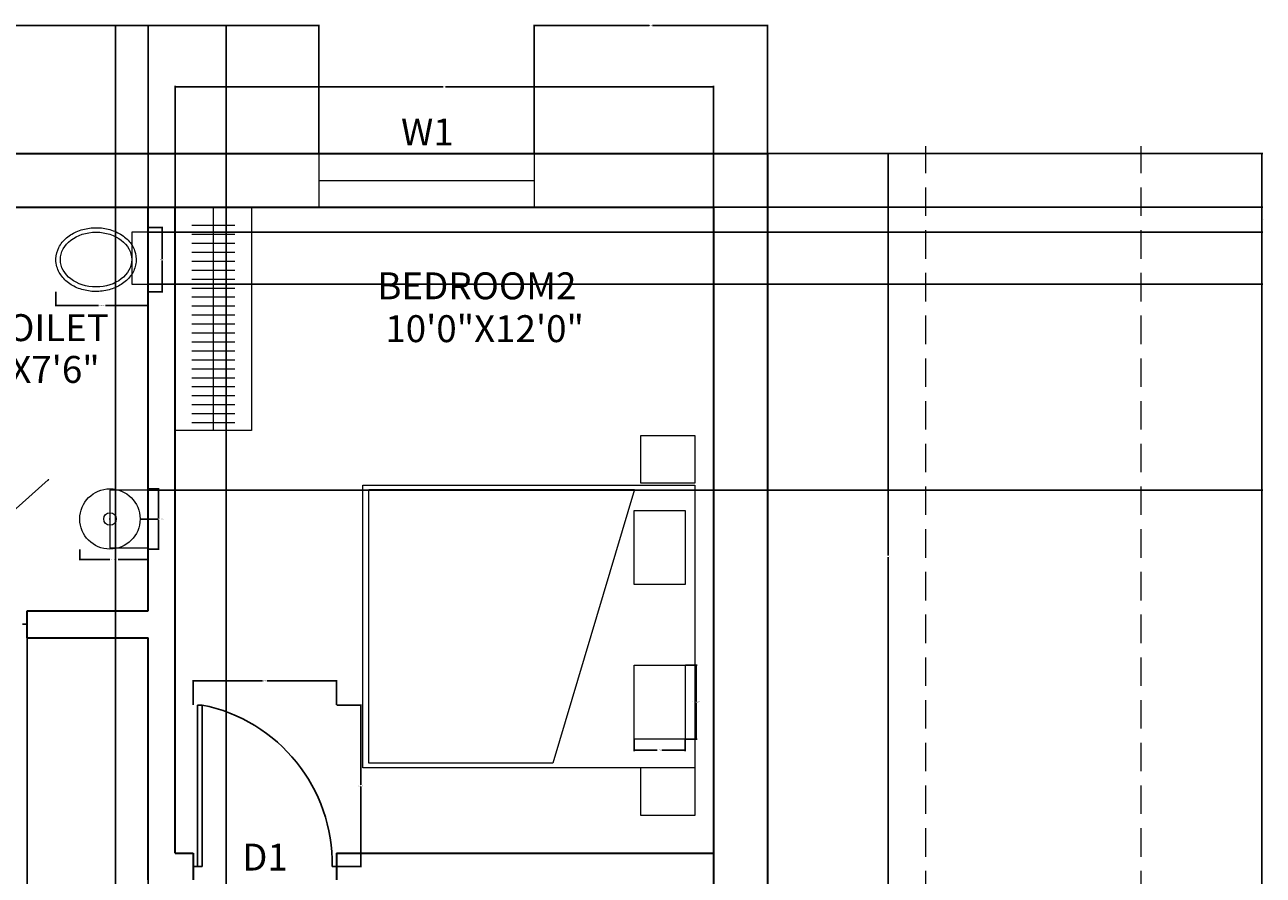
# Model space of a CAD drawing. Units: inches. Extents: x 2906 to 3403, y 1614 to 2150.
# Tile 4 of 4: x 3127 to 3403, y 1960 to 2150. Entities that reach past the tile are written whole.
import ezdxf

# ---------------------------------------------------------------- set-up
doc = ezdxf.new("R2010")
doc.units = ezdxf.units.IN
doc.linetypes.add('DASHED2', pattern=[9.525, 6.35, -3.175])
for name, color, linetype, lineweight in [('A-ANNO-DIMS', 2, 'Continuous', 18), ('A-ANNO-TEXT', 220, 'Continuous', 18), ('A-AREA-IDEN', 220, 'Continuous', 25), ('A-DOOR', 40, 'Continuous', 25), ('A-FLOR-CASE', 121, 'Continuous', 18), ('A-FLOR-FIXT', 121, 'Continuous', 18), ('A-FURN', 121, 'Continuous', 18), ('A-GLAZ', 2, 'Continuous', 18), ('A-WALL', 191, 'Continuous', 35), ('C-ROAD', 255, 'DASHED2', 18)]:
    doc.layers.add(name, color=color, linetype=linetype, lineweight=lineweight)
doc.styles.get("Standard").update_dxf_attribs({"font": 'arial.ttf'})
doc.dimstyles.get("Standard").update_dxf_attribs({"dimtxt": 0.18, "dimasz": 0.18, "dimexe": 0.18, "dimexo": 0.0625, "dimgap": 0.09, "dimtad": 0, "dimtih": 1, "dimtoh": 1, "dimdec": 4, "dimzin": 0, "dimdsep": 46, "dimtxsty": 'Standard', "dimcen": 0.09, "dimadec": 0, "dimazin": 0, "dimtfac": 1, "dimtdec": 4, "dimtofl": 0, "dimtmove": 0, "dimatfit": 3, "dimfxl": 1, "dimtolj": 1, "dimtzin": 0, "dimarcsym": 0})

# ---------------------------------------------------------------- blocks, each defined once
blk = doc.blocks.new('DOOR-SWING-36')
for p, q in [((36, 32), (36, 31)), ((0, 1), (0, 2)), ((0, 2), (36, 2)), ((36, 1), (0, 1)), ((36, 2), (36, 1)), ((36, 0), (36, 1))]:
    blk.add_line(p, q)
blk.add_arc((35.31, -4.99), 36, 88.9084, 168.7983)
blk = doc.blocks.new('WINDOW-48')
for p, q in [((0, 12), (0, 0)), ((48, 12), (48, 0)), ((0, 6), (48, 6))]:
    blk.add_line(p, q)
blk = doc.blocks.new('WC-FLOOR')
blk.add_lwpolyline([(20.57, 13.25), (16.9, 13.25), (16.9, 1.66), (20.57, 1.66)], close=True)
blk.add_ellipse((8.95, 7.12), major_axis=(-7.95, 0), ratio=0.769471)
blk.add_open_spline([(0, 7.12), (0, 6.57), (0.08, 6.02), (0.48, 4.65), (0.93, 3.84), (2.12, 2.43), (2.86, 1.82), (4.56, 0.85), (5.51, 0.49), (7.5, 0.04), (8.54, -0.04), (10.6, 0.07), (11.62, 0.27), (13.52, 0.93), (14.4, 1.4), (15.92, 2.56), (16.56, 3.25), (17.49, 4.8), (17.78, 5.66), (17.96, 7.41), (17.85, 8.3), (17.23, 9.97), (16.74, 10.74), (15.46, 12.09), (14.67, 12.67), (12.92, 13.56), (11.94, 13.88), (9.93, 14.24), (8.88, 14.28), (6.83, 14.08), (5.83, 13.84), (3.97, 13.1), (3.12, 12.59), (1.68, 11.37), (1.09, 10.64), (0.26, 9.05), (0.03, 8.17), (0, 7.24), (0, 7.18), (0, 7.12)], degree=3, knots=[0, 0, 0, 0, 0.221105, 0.221105, 0.576279, 0.576279, 0.931454, 0.931454, 1.286628, 1.286628, 1.641803, 1.641803, 1.996977, 1.996977, 2.352152, 2.352152, 2.707326, 2.707326, 3.062501, 3.062501, 3.417675, 3.417675, 3.77285, 3.77285, 4.128024, 4.128024, 4.483198, 4.483198, 4.838373, 4.838373, 5.193547, 5.193547, 5.548722, 5.548722, 5.903896, 5.903896, 6.259071, 6.259071, 6.283185, 6.283185, 6.283185, 6.283185])
blk = doc.blocks.new('LAVATORY-WALL')
blk.add_lwpolyline([(15.24, 13.17), (6.72, 13.17), (6.72, 0.27), (15.24, 0.27)], close=True)
for radius in [6.72, 1.39]:
    blk.add_circle((6.72, 6.72), radius)
blk = doc.blocks.new('WARDROBE-RAIL')
for p, q in [((4.8, 49.77), (4.8, 0)), ((0, 45.77), (9.61, 45.77)), ((0, 43.77), (9.61, 43.77)), ((0, 41.77), (9.61, 41.77)), ((0, 39.77), (9.61, 39.77)), ((0, 37.77), (9.61, 37.77)), ((0, 35.77), (9.61, 35.77)), ((0, 33.77), (9.61, 33.77)), ((0, 31.77), (9.61, 31.77)), ((0, 29.77), (9.61, 29.77)), ((0, 27.77), (9.61, 27.77)), ((0, 25.77), (9.61, 25.77)), ((0, 23.77), (9.61, 23.77)), ((0, 21.77), (9.61, 21.77)), ((0, 19.77), (9.61, 19.77)), ((0, 17.77), (9.61, 17.77)), ((0, 15.77), (9.61, 15.77)), ((0, 13.77), (9.61, 13.77)), ((0, 11.77), (9.61, 11.77)), ((0, 9.77), (9.61, 9.77)), ((0, 7.77), (9.61, 7.77)), ((0, 5.77), (9.61, 5.77)), ((0, 3.77), (9.61, 3.77)), ((0, 1.77), (9.61, 1.77))]:
    blk.add_line(p, q)
blk = doc.blocks.new('NIGHTSTAND')
blk.add_lwpolyline([(0, 10.63), (12.01, 10.63), (12.01, 0), (0, 0)], close=True)
blk = doc.blocks.new('BED-PILLOW')
blk.add_lwpolyline([(0, 16.48), (11.36, 16.48), (11.36, 0), (0, 0)], close=True)
blk = doc.blocks.new('*D16')
at = {"layer": 'A-ANNO-DIMS', "color": 0, "lineweight": -2, "transparency": 16777216}
for p, q in [((3274.36, 2007.13), (3276.95, 2007.13)), ((3276.77, 2006.95), (3276.77, 1999.07)), ((3276.77, 1990.83), (3276.77, 1998.71)), ((3274.36, 1990.65), (3276.95, 1990.65))]:
    blk.add_line(p, q, dxfattribs=at)
at = {"layer": 'A-ANNO-DIMS', "color": 0, "transparency": 16777216}
for points in [[(3276.74, 2006.95), (3276.8, 2006.95), (3276.77, 2007.13)], [(3276.74, 1990.83), (3276.8, 1990.83), (3276.77, 1990.65)]]:
    blk.add_solid(points, dxfattribs=at)
at = {"layer": 'Defpoints', "color": 0, "transparency": 16777216}
for p in [(3274.3, 2007.13), (3276.77, 2007.13), (3274.3, 1990.65)]:
    blk.add_point(p, dxfattribs=at)
at = {"layer": 'A-ANNO-DIMS', "color": 0, "transparency": 16777216, "insert": (3276.77, 1998.89), "char_height": 0.18, "attachment_point": 5}
blk.add_mtext('\\A1;PILLOW 16 TYP.', dxfattribs=at)
blk = doc.blocks.new('*D17')
at = {"layer": 'A-ANNO-DIMS', "color": 0, "lineweight": -2, "transparency": 16777216}
for p, q in [((3262.93, 1990.59), (3262.93, 1988)), ((3274.3, 1990.59), (3274.3, 1988)), ((3263.11, 1988.18), (3268.1, 1988.18)), ((3274.12, 1988.18), (3269.14, 1988.18))]:
    blk.add_line(p, q, dxfattribs=at)
at = {"layer": 'A-ANNO-DIMS', "color": 0, "transparency": 16777216}
for points in [[(3263.11, 1988.21), (3263.11, 1988.15), (3262.93, 1988.18)], [(3274.12, 1988.21), (3274.12, 1988.15), (3274.3, 1988.18)]]:
    blk.add_solid(points, dxfattribs=at)
at = {"layer": 'Defpoints', "color": 0, "transparency": 16777216}
for p in [(3262.93, 1990.65), (3274.3, 1990.65), (3274.3, 1988.18)]:
    blk.add_point(p, dxfattribs=at)
at = {"layer": 'A-ANNO-DIMS', "color": 0, "transparency": 16777216, "insert": (3268.62, 1988.18), "char_height": 0.18, "attachment_point": 5}
blk.add_mtext('\\A1;11 TYP.', dxfattribs=at)
blk = doc.blocks.new('*D20')
at = {"layer": 'A-ANNO-DIMS', "color": 0, "lineweight": -2, "transparency": 16777216}
for p, q in [((3196.7, 1998.25), (3202.21, 1998.25)), ((3202.03, 1998.07), (3202.03, 1980.44)), ((3202.03, 1962.43), (3202.03, 1980.07)), ((3196.7, 1962.25), (3202.21, 1962.25))]:
    blk.add_line(p, q, dxfattribs=at)
at = {"layer": 'A-ANNO-DIMS', "color": 0, "transparency": 16777216}
for points in [[(3202, 1998.07), (3202.06, 1998.07), (3202.03, 1998.25)], [(3202, 1962.43), (3202.06, 1962.43), (3202.03, 1962.25)]]:
    blk.add_solid(points, dxfattribs=at)
at = {"layer": 'Defpoints', "color": 0, "transparency": 16777216}
for p in [(3196.63, 1998.25), (3196.63, 1962.25), (3202.03, 1962.25)]:
    blk.add_point(p, dxfattribs=at)
at = {"layer": 'A-ANNO-DIMS', "color": 0, "transparency": 16777216, "insert": (3202.03, 1980.25), "char_height": 0.18, "attachment_point": 5}
blk.add_mtext('\\A1;D1 36 TYP.', dxfattribs=at)
blk = doc.blocks.new('*D21')
at = {"layer": 'A-ANNO-DIMS', "color": 0, "lineweight": -2, "transparency": 16777216}
for p, q in [((3164.63, 1998.32), (3164.63, 2003.83)), ((3196.63, 1998.32), (3196.63, 2003.83)), ((3164.81, 2003.65), (3180.1, 2003.65)), ((3196.45, 2003.65), (3181.16, 2003.65))]:
    blk.add_line(p, q, dxfattribs=at)
at = {"layer": 'A-ANNO-DIMS', "color": 0, "transparency": 16777216}
for points in [[(3164.81, 2003.68), (3164.81, 2003.62), (3164.63, 2003.65)], [(3196.45, 2003.68), (3196.45, 2003.62), (3196.63, 2003.65)]]:
    blk.add_solid(points, dxfattribs=at)
at = {"layer": 'Defpoints', "color": 0, "transparency": 16777216}
for p in [(3196.63, 2003.65), (3164.63, 1998.25), (3196.63, 1998.25)]:
    blk.add_point(p, dxfattribs=at)
at = {"layer": 'A-ANNO-DIMS', "color": 0, "transparency": 16777216, "insert": (3180.63, 2003.65), "char_height": 0.18, "attachment_point": 5}
blk.add_mtext('\\A1;32 TYP.', dxfattribs=at)
blk = doc.blocks.new('*D26')
at = {"layer": 'A-ANNO-DIMS', "color": 0, "lineweight": -2, "transparency": 16777216}
for p, q in [((3134.07, 2090.37), (3134.07, 2087.17)), ((3154.63, 2090.37), (3154.63, 2087.17)), ((3134.25, 2087.35), (3143.57, 2087.35)), ((3154.45, 2087.35), (3145.13, 2087.35))]:
    blk.add_line(p, q, dxfattribs=at)
at = {"layer": 'A-ANNO-DIMS', "color": 0, "transparency": 16777216}
for points in [[(3134.25, 2087.38), (3134.25, 2087.32), (3134.07, 2087.35)], [(3154.45, 2087.38), (3154.45, 2087.32), (3154.63, 2087.35)]]:
    blk.add_solid(points, dxfattribs=at)
at = {"layer": 'Defpoints', "color": 0, "transparency": 16777216}
for p in [(3134.07, 2090.43), (3154.63, 2090.43), (3154.63, 2087.35)]:
    blk.add_point(p, dxfattribs=at)
at = {"layer": 'A-ANNO-DIMS', "color": 0, "transparency": 16777216, "insert": (3144.35, 2087.35), "char_height": 0.18, "attachment_point": 5}
blk.add_mtext('\\A1;WC 21 TYP.', dxfattribs=at)
blk = doc.blocks.new('*D27')
at = {"layer": 'A-ANNO-DIMS', "color": 0, "lineweight": -2, "transparency": 16777216}
for p, q in [((3154.7, 2104.76), (3157.9, 2104.76)), ((3157.72, 2104.58), (3157.72, 2097.78)), ((3157.72, 2090.61), (3157.72, 2097.42)), ((3154.7, 2090.43), (3157.9, 2090.43))]:
    blk.add_line(p, q, dxfattribs=at)
at = {"layer": 'A-ANNO-DIMS', "color": 0, "transparency": 16777216}
for points in [[(3157.69, 2104.58), (3157.75, 2104.58), (3157.72, 2104.76)], [(3157.69, 2090.61), (3157.75, 2090.61), (3157.72, 2090.43)]]:
    blk.add_solid(points, dxfattribs=at)
at = {"layer": 'Defpoints', "color": 0, "transparency": 16777216}
for p in [(3154.63, 2104.76), (3157.72, 2104.76), (3154.63, 2090.43)]:
    blk.add_point(p, dxfattribs=at)
at = {"layer": 'A-ANNO-DIMS', "color": 0, "transparency": 16777216, "insert": (3157.72, 2097.6), "char_height": 0.18, "attachment_point": 5}
blk.add_mtext('\\A1;14 TYP.', dxfattribs=at)
blk = doc.blocks.new('*D28')
at = {"layer": 'A-ANNO-DIMS', "color": 0, "lineweight": -2, "transparency": 16777216}
for p, q in [((3139.39, 2032.96), (3139.39, 2030.56)), ((3154.63, 2032.96), (3154.63, 2030.56)), ((3139.57, 2030.74), (3146.08, 2030.74)), ((3154.45, 2030.74), (3147.95, 2030.74))]:
    blk.add_line(p, q, dxfattribs=at)
at = {"layer": 'A-ANNO-DIMS', "color": 0, "transparency": 16777216}
for points in [[(3139.57, 2030.77), (3139.57, 2030.71), (3139.39, 2030.74)], [(3154.45, 2030.77), (3154.45, 2030.71), (3154.63, 2030.74)]]:
    blk.add_solid(points, dxfattribs=at)
at = {"layer": 'Defpoints', "color": 0, "transparency": 16777216}
for p in [(3139.39, 2033.03), (3154.63, 2033.03), (3154.63, 2030.74)]:
    blk.add_point(p, dxfattribs=at)
at = {"layer": 'A-ANNO-DIMS', "color": 0, "transparency": 16777216, "insert": (3147.01, 2030.74), "char_height": 0.18, "attachment_point": 5}
blk.add_mtext('\\A1;BASIN 15 TYP.', dxfattribs=at)
blk = doc.blocks.new('*D29')
at = {"layer": 'A-ANNO-DIMS', "color": 0, "lineweight": -2, "transparency": 16777216}
for p, q in [((3154.7, 2046.46), (3157.1, 2046.46)), ((3156.92, 2046.28), (3156.92, 2039.93)), ((3156.92, 2033.21), (3156.92, 2039.56)), ((3154.7, 2033.03), (3157.1, 2033.03))]:
    blk.add_line(p, q, dxfattribs=at)
at = {"layer": 'A-ANNO-DIMS', "color": 0, "transparency": 16777216}
for points in [[(3156.89, 2046.28), (3156.95, 2046.28), (3156.92, 2046.46)], [(3156.89, 2033.21), (3156.95, 2033.21), (3156.92, 2033.03)]]:
    blk.add_solid(points, dxfattribs=at)
at = {"layer": 'Defpoints', "color": 0, "transparency": 16777216}
for p in [(3154.63, 2046.46), (3156.92, 2046.46), (3154.63, 2033.03)]:
    blk.add_point(p, dxfattribs=at)
at = {"layer": 'A-ANNO-DIMS', "color": 0, "transparency": 16777216, "insert": (3156.92, 2039.74), "char_height": 0.18, "attachment_point": 5}
blk.add_mtext('\\A1;13 TYP.', dxfattribs=at)
blk = doc.blocks.new('*D41')
at = {"layer": 'A-ANNO-DIMS', "color": 0, "lineweight": -2, "transparency": 16777216}
for p, q in [((3292.7, 2121.25), (3403.01, 2121.25)), ((3402.83, 2121.07), (3402.83, 1881.44)), ((3402.83, 1641.43), (3402.83, 1881.07)), ((3292.7, 1641.25), (3403.01, 1641.25))]:
    blk.add_line(p, q, dxfattribs=at)
at = {"layer": 'A-ANNO-DIMS', "color": 0, "transparency": 16777216}
for points in [[(3402.8, 2121.07), (3402.86, 2121.07), (3402.83, 2121.25)], [(3402.8, 1641.43), (3402.86, 1641.43), (3402.83, 1641.25)]]:
    blk.add_solid(points, dxfattribs=at)
at = {"layer": 'Defpoints', "color": 0, "transparency": 16777216}
for p in [(3292.63, 2121.25), (3402.83, 2121.25), (3292.63, 1641.25)]:
    blk.add_point(p, dxfattribs=at)
at = {"layer": 'A-ANNO-DIMS', "color": 0, "transparency": 16777216, "insert": (3402.83, 1881.25), "char_height": 0.18, "attachment_point": 5}
blk.add_mtext('\\A1;480', dxfattribs=at)
blk = doc.blocks.new('*D43')
at = {"layer": 'A-ANNO-DIMS', "color": 0, "lineweight": -2, "transparency": 16777216}
for p, q in [((3025.57, 2121.32), (3025.57, 2149.96)), ((3025.75, 2149.78), (3108.75, 2149.78)), ((3192.49, 2149.78), (3109.49, 2149.78)), ((3192.67, 2121.32), (3192.67, 2149.96))]:
    blk.add_line(p, q, dxfattribs=at)
at = {"layer": 'A-ANNO-DIMS', "color": 0, "transparency": 16777216}
for points in [[(3025.75, 2149.81), (3025.75, 2149.75), (3025.57, 2149.78)], [(3192.49, 2149.81), (3192.49, 2149.75), (3192.67, 2149.78)]]:
    blk.add_solid(points, dxfattribs=at)
at = {"layer": 'Defpoints', "color": 0, "transparency": 16777216}
for p in [(3192.67, 2149.78), (3025.57, 2121.25), (3192.67, 2121.25)]:
    blk.add_point(p, dxfattribs=at)
at = {"layer": 'A-ANNO-DIMS', "color": 0, "transparency": 16777216, "insert": (3109.12, 2149.78), "char_height": 0.18, "attachment_point": 5}
blk.add_mtext('\\A1;167.1', dxfattribs=at)
blk = doc.blocks.new('*D44')
at = {"layer": 'A-ANNO-DIMS', "color": 0, "lineweight": -2, "transparency": 16777216}
for p, q in [((3240.67, 2121.32), (3240.67, 2149.96)), ((3240.85, 2149.78), (3266.26, 2149.78)), ((3292.45, 2149.78), (3267.05, 2149.78)), ((3292.63, 2121.32), (3292.63, 2149.96))]:
    blk.add_line(p, q, dxfattribs=at)
at = {"layer": 'A-ANNO-DIMS', "color": 0, "transparency": 16777216}
for points in [[(3240.85, 2149.81), (3240.85, 2149.75), (3240.67, 2149.78)], [(3292.45, 2149.81), (3292.45, 2149.75), (3292.63, 2149.78)]]:
    blk.add_solid(points, dxfattribs=at)
at = {"layer": 'Defpoints', "color": 0, "transparency": 16777216}
for p in [(3292.63, 2149.78), (3240.67, 2121.25), (3292.63, 2121.25)]:
    blk.add_point(p, dxfattribs=at)
at = {"layer": 'A-ANNO-DIMS', "color": 0, "transparency": 16777216, "insert": (3266.65, 2149.78), "char_height": 0.18, "attachment_point": 5}
blk.add_mtext('\\A1;51.96', dxfattribs=at)
blk = doc.blocks.new('*D46')
at = {"layer": 'A-ANNO-DIMS', "color": 0, "lineweight": -2, "transparency": 16777216}
for p, q in [((3094.63, 2109.32), (3094.63, 2149.96)), ((3094.81, 2149.78), (3124.41, 2149.78)), ((3154.45, 2149.78), (3124.85, 2149.78)), ((3154.63, 2109.32), (3154.63, 2149.96))]:
    blk.add_line(p, q, dxfattribs=at)
at = {"layer": 'A-ANNO-DIMS', "color": 0, "transparency": 16777216}
for points in [[(3094.81, 2149.81), (3094.81, 2149.75), (3094.63, 2149.78)], [(3154.45, 2149.81), (3154.45, 2149.75), (3154.63, 2149.78)]]:
    blk.add_solid(points, dxfattribs=at)
at = {"layer": 'Defpoints', "color": 0, "transparency": 16777216}
for p in [(3154.63, 2149.78), (3094.63, 2109.25), (3154.63, 2109.25)]:
    blk.add_point(p, dxfattribs=at)
at = {"layer": 'A-ANNO-DIMS', "color": 0, "transparency": 16777216, "insert": (3124.63, 2149.78), "char_height": 0.18, "attachment_point": 5}
blk.add_mtext('\\A1;60', dxfattribs=at)
blk = doc.blocks.new('*D47')
at = {"layer": 'A-ANNO-DIMS', "color": 0, "lineweight": -2, "transparency": 16777216}
for p, q in [((3160.63, 2109.32), (3160.63, 2136.33)), ((3280.63, 2109.32), (3280.63, 2136.33)), ((3160.81, 2136.15), (3220.35, 2136.15)), ((3280.45, 2136.15), (3220.91, 2136.15))]:
    blk.add_line(p, q, dxfattribs=at)
at = {"layer": 'A-ANNO-DIMS', "color": 0, "transparency": 16777216}
for points in [[(3160.81, 2136.18), (3160.81, 2136.12), (3160.63, 2136.15)], [(3280.45, 2136.18), (3280.45, 2136.12), (3280.63, 2136.15)]]:
    blk.add_solid(points, dxfattribs=at)
at = {"layer": 'Defpoints', "color": 0, "transparency": 16777216}
for p in [(3280.63, 2136.15), (3160.63, 2109.25), (3280.63, 2109.25)]:
    blk.add_point(p, dxfattribs=at)
at = {"layer": 'A-ANNO-DIMS', "color": 0, "transparency": 16777216, "insert": (3220.63, 2136.15), "char_height": 0.18, "attachment_point": 5}
blk.add_mtext('\\A1;120', dxfattribs=at)
blk = doc.blocks.new('*D66')
at = {"layer": 'A-ANNO-DIMS', "color": 0, "lineweight": -2, "transparency": 16777216}
for p, q in [((3292.7, 2121.25), (3319.71, 2121.25)), ((3319.53, 2121.07), (3319.53, 2031.6)), ((3319.53, 1941.76), (3319.53, 2031.24)), ((3292.7, 1941.58), (3319.71, 1941.58))]:
    blk.add_line(p, q, dxfattribs=at)
at = {"layer": 'A-ANNO-DIMS', "color": 0, "transparency": 16777216}
for points in [[(3319.5, 2121.07), (3319.56, 2121.07), (3319.53, 2121.25)], [(3319.5, 1941.76), (3319.56, 1941.76), (3319.53, 1941.58)]]:
    blk.add_solid(points, dxfattribs=at)
at = {"layer": 'Defpoints', "color": 0, "transparency": 16777216}
for p in [(3292.63, 2121.25), (3292.63, 1941.58), (3319.53, 1941.58)]:
    blk.add_point(p, dxfattribs=at)
at = {"layer": 'A-ANNO-DIMS', "color": 0, "transparency": 16777216, "insert": (3319.53, 2031.42), "char_height": 0.18, "attachment_point": 5}
blk.add_mtext('\\A1;179.67', dxfattribs=at)
blk = doc.blocks.new('*D75')
at = {"layer": 'A-ANNO-DIMS', "color": 0, "lineweight": -2, "transparency": 16777216}
for p, q in [((3127.63, 2013.19), (3127.63, 1613.51)), ((3154.63, 2013.19), (3154.63, 1613.51)), ((3127.81, 1613.69), (3140.91, 1613.69)), ((3154.45, 1613.69), (3141.35, 1613.69))]:
    blk.add_line(p, q, dxfattribs=at)
at = {"layer": 'A-ANNO-DIMS', "color": 0, "transparency": 16777216}
for points in [[(3127.81, 1613.72), (3127.81, 1613.66), (3127.63, 1613.69)], [(3154.45, 1613.72), (3154.45, 1613.66), (3154.63, 1613.69)]]:
    blk.add_solid(points, dxfattribs=at)
at = {"layer": 'Defpoints', "color": 0, "transparency": 16777216}
for p in [(3127.63, 2013.25), (3154.63, 2013.25), (3154.63, 1613.69)]:
    blk.add_point(p, dxfattribs=at)
at = {"layer": 'A-ANNO-DIMS', "color": 0, "transparency": 16777216, "insert": (3141.13, 1613.69), "char_height": 0.18, "attachment_point": 5}
blk.add_mtext('\\A1;27', dxfattribs=at)
blk = doc.blocks.new('*D76')
at = {"layer": 'A-ANNO-DIMS', "color": 0, "lineweight": -2, "transparency": 16777216}
for p, q in [((3154.7, 2109.25), (3403.01, 2109.25)), ((3402.83, 2109.07), (3402.83, 2106.67)), ((3402.83, 2103.91), (3402.83, 2106.31)), ((3154.7, 2103.73), (3403.01, 2103.73))]:
    blk.add_line(p, q, dxfattribs=at)
at = {"layer": 'A-ANNO-DIMS', "color": 0, "transparency": 16777216}
for points in [[(3402.8, 2109.07), (3402.86, 2109.07), (3402.83, 2109.25)], [(3402.8, 2103.91), (3402.86, 2103.91), (3402.83, 2103.73)]]:
    blk.add_solid(points, dxfattribs=at)
at = {"layer": 'Defpoints', "color": 0, "transparency": 16777216}
for p in [(3154.63, 2109.25), (3154.63, 2103.73), (3402.83, 2103.73)]:
    blk.add_point(p, dxfattribs=at)
at = {"layer": 'A-ANNO-DIMS', "color": 0, "transparency": 16777216, "insert": (3402.83, 2106.49), "char_height": 0.18, "attachment_point": 5}
blk.add_mtext('\\A1;5.526', dxfattribs=at)
blk = doc.blocks.new('*D77')
at = {"layer": 'A-ANNO-DIMS', "color": 0, "lineweight": -2, "transparency": 16777216}
for p, q in [((3154.7, 2092.13), (3403.01, 2092.13)), ((3402.83, 2091.95), (3402.83, 2069.35)), ((3402.83, 2046.37), (3402.83, 2068.98)), ((3154.7, 2046.19), (3403.01, 2046.19))]:
    blk.add_line(p, q, dxfattribs=at)
at = {"layer": 'A-ANNO-DIMS', "color": 0, "transparency": 16777216}
for points in [[(3402.8, 2091.95), (3402.86, 2091.95), (3402.83, 2092.13)], [(3402.8, 2046.37), (3402.86, 2046.37), (3402.83, 2046.19)]]:
    blk.add_solid(points, dxfattribs=at)
at = {"layer": 'Defpoints', "color": 0, "transparency": 16777216}
for p in [(3154.63, 2092.13), (3154.63, 2046.19), (3402.83, 2046.19)]:
    blk.add_point(p, dxfattribs=at)
at = {"layer": 'A-ANNO-DIMS', "color": 0, "transparency": 16777216, "insert": (3402.83, 2069.16), "char_height": 0.18, "attachment_point": 5}
blk.add_mtext('\\A1;45.94', dxfattribs=at)
blk = doc.blocks.new('*D78')
at = {"layer": 'A-ANNO-DIMS', "color": 0, "lineweight": -2, "transparency": 16777216}
for p, q in [((3147.32, 1912.74), (3147.32, 2149.96)), ((3147.5, 2149.78), (3159.2, 2149.78)), ((3171.82, 2149.78), (3160.13, 2149.78)), ((3172, 1912.74), (3172, 2149.96))]:
    blk.add_line(p, q, dxfattribs=at)
at = {"layer": 'A-ANNO-DIMS', "color": 0, "transparency": 16777216}
for points in [[(3147.5, 2149.81), (3147.5, 2149.75), (3147.32, 2149.78)], [(3171.82, 2149.81), (3171.82, 2149.75), (3172, 2149.78)]]:
    blk.add_solid(points, dxfattribs=at)
at = {"layer": 'Defpoints', "color": 0, "transparency": 16777216}
for p in [(3172, 2149.78), (3147.32, 1912.68), (3172, 1912.68)]:
    blk.add_point(p, dxfattribs=at)
at = {"layer": 'A-ANNO-DIMS', "color": 0, "transparency": 16777216, "insert": (3159.66, 2149.78), "char_height": 0.18, "attachment_point": 5}
blk.add_mtext('\\A1;24.675', dxfattribs=at)
blk = doc.blocks.new('*D82')
at = {"layer": 'A-ANNO-DIMS', "color": 0, "lineweight": -2, "transparency": 16777216}
for p, q in [((3132.31, 2048.51), (3119.07, 2036.59)), ((3132.49, 2048.51), (3132.31, 2048.51)), ((3096.54, 2016.4), (3096.72, 2016.4)), ((3096.63, 2016.31), (3096.63, 2016.49))]:
    blk.add_line(p, q, dxfattribs=at)
at = {"layer": 'A-ANNO-DIMS', "color": 0, "transparency": 16777216}
blk.add_solid([(3119.05, 2036.62), (3119.09, 2036.57), (3118.93, 2036.47)], dxfattribs=at)
at = {"layer": 'Defpoints', "color": 0, "transparency": 16777216}
for p in [(3118.93, 2036.47), (3096.63, 2016.4)]:
    blk.add_point(p, dxfattribs=at)
at = {"layer": 'A-ANNO-DIMS', "color": 0, "transparency": 16777216, "insert": (3132.8, 2048.51), "char_height": 0.18, "attachment_point": 5}
blk.add_mtext('\\A1;R30', dxfattribs=at)
blk = doc.blocks.new('*D84')
at = {"layer": 'A-ANNO-DIMS', "color": 0, "lineweight": -2, "transparency": 16777216}
for p, q in [((3146.02, 2039.74), (3146.2, 2039.74)), ((3146.11, 2039.65), (3146.11, 2039.83)), ((3156.85, 2039.74), (3153, 2039.74))]:
    blk.add_line(p, q, dxfattribs=at)
at = {"layer": 'A-ANNO-DIMS', "color": 0, "transparency": 16777216}
blk.add_solid([(3153, 2039.77), (3153, 2039.71), (3152.82, 2039.74)], dxfattribs=at)
at = {"layer": 'Defpoints', "color": 0, "transparency": 16777216}
for p in [(3139.39, 2039.74), (3152.82, 2039.74)]:
    blk.add_point(p, dxfattribs=at)
at = {"layer": 'A-ANNO-DIMS', "color": 0, "transparency": 16777216, "insert": (3157.61, 2039.74), "char_height": 0.18, "attachment_point": 5}
blk.add_mtext('\\A1;2X ∅13.433', dxfattribs=at)

msp = doc.modelspace()

# ---------------------------------------------------------------- linework, layer by layer
at = {"layer": 'A-DOOR'}
msp.add_line((3127.6325, 2016.254), (3126.6325, 2016.254), dxfattribs=at)
at = {"layer": 'A-FLOR-CASE'}
for p, q in [((3160.6325, 2109.254), (3177.6325, 2109.254)), ((3177.6325, 2109.254), (3177.6325, 2059.4818)), ((3177.6325, 2059.4818), (3160.6325, 2059.4818))]:
    msp.add_line(p, q, dxfattribs=at)
at = {"layer": 'A-FURN'}
for p, q in [((3203.8046, 1985.2873), (3203.8046, 2046.2873)), ((3203.8046, 2046.2873), (3263.0104, 2046.2873)), ((3263.0104, 2046.2873), (3244.8046, 1985.2873)), ((3244.8046, 1985.2873), (3203.8046, 1985.2873))]:
    msp.add_line(p, q, dxfattribs=at)
msp.add_lwpolyline([(3276.4421, 1984.2873), (3202.4421, 1984.2873), (3202.4421, 2047.2873), (3276.4421, 2047.2873)], close=True, dxfattribs=at)
at = {"layer": 'A-WALL'}
for p, q in [((2944.6325, 2109.254), (3280.6325, 2109.254)), ((3154.6325, 2019.254), (3154.6325, 2109.254)), ((3160.6325, 1965.254), (3160.6325, 2109.254)), ((3280.6325, 2109.254), (3280.6325, 1701.254)), ((3127.6325, 2013.254), (3127.6325, 2019.254)), ((3127.6325, 2019.254), (3154.6325, 2019.254)), ((3127.6325, 2013.254), (3154.6325, 2013.254)), ((3154.6325, 1959.254), (3154.6325, 2013.254)), ((3160.6325, 1965.254), (3164.6325, 1965.254)), ((3164.6325, 1965.254), (3164.6325, 1959.254)), ((3196.6325, 1965.254), (3196.6325, 1959.254)), ((3196.6325, 1965.254), (3280.6325, 1965.254))]:
    msp.add_line(p, q, dxfattribs=at)
msp.add_lwpolyline([(3022.1668, 1641.254), (2932.6325, 1641.254), (2932.6325, 2121.254), (3292.6325, 2121.254), (3292.6325, 1689.254)], dxfattribs=at)
at = {"layer": 'C-ROAD'}
for p, q in [((3327.9288, 1640.586), (3327.9288, 2122.8771)), ((3375.9288, 1640.586), (3375.9288, 2122.8771))]:
    msp.add_line(p, q, dxfattribs=at)

# ---------------------------------------------------------------- block references
at = {"layer": 'A-DOOR', "rotation": 269.9999999999988}
msp.add_blockref('DOOR-SWING-36', (3164.6326, 1998.2535), dxfattribs=at)
at = {"layer": 'A-FLOR-CASE'}
msp.add_blockref('WARDROBE-RAIL', (3164.334, 2059.482), dxfattribs=at)
at = {"layer": 'A-FLOR-FIXT'}
for name, p in [('WC-FLOOR', (3134.066, 2090.474)), ('LAVATORY-WALL', (3139.391, 2033.027))]:
    msp.add_blockref(name, p, dxfattribs=at)
at = {"layer": 'A-FURN'}
for name, p in [('NIGHTSTAND', (3264.432, 2047.7191)), ('BED-PILLOW', (3262.9331, 2025.159)), ('BED-PILLOW', (3262.9331, 1990.6499)), ('NIGHTSTAND', (3264.432, 1973.659))]:
    msp.add_blockref(name, p, dxfattribs=at)
at = {"layer": 'A-GLAZ'}
msp.add_blockref('WINDOW-48', (3192.6745, 2109.254), dxfattribs=at)

# ---------------------------------------------------------------- texts
at = {"layer": 'A-ANNO-TEXT'}
for tag, p in [('W1', (3210.9872, 2123.0422)), ('D1', (3175.5801, 1961.3438))]:
    msp.add_attdef(tag, p, '', height=6, dxfattribs=at)
at = {"layer": 'A-AREA-IDEN'}
for tag, p in [('BEDROOM2', (3205.7031, 2088.7373)), ('ATT.TOILET', (3101.2536, 2079.4131)), ('10\'0"X12\'0"', (3207.4877, 2079.1858)), ('4\'6"X7\'6"', (3108.6552, 2070.1006))]:
    msp.add_attdef(tag, p, '', height=6, dxfattribs=at)

# ---------------------------------------------------------------- dimensions: what is measured, and where the dimension line sits
at = {"layer": 'A-ANNO-DIMS'}
for base, p1, p2, override, picture, middle in [((3192.6748, 2149.7771), (3025.5663, 2121.254), (3192.6748, 2121.254), {"dimdec": 1, "dimlfac": 1, "dimrnd": 0, "dimzin": 0, "dimdsep": 46, "dimlunit": 2}, '*D43', (3109.1205, 2149.7771)), ((3154.6325, 2149.7771), (3094.6325, 2109.254), (3154.6325, 2109.254), {"dimdec": 0, "dimlfac": 1, "dimrnd": 0, "dimzin": 0, "dimdsep": 46, "dimlunit": 2}, '*D46', (3124.6325, 2149.7771)), ((3171.9988, 2149.7771), (3147.3239, 1912.6757), (3171.9988, 1912.6757), {"dimdec": 3, "dimlfac": 1, "dimrnd": 0, "dimzin": 0, "dimdsep": 46, "dimlunit": 2}, '*D78', (3159.6614, 2149.7771)), ((3292.6325, 2149.7771), (3240.6748, 2121.254), (3292.6325, 2121.254), {"dimdec": 2, "dimlfac": 1, "dimrnd": 0, "dimzin": 0, "dimdsep": 46, "dimlunit": 2}, '*D44', (3266.6536, 2149.7771)), ((3280.6325, 2136.154), (3160.6325, 2109.254), (3280.6325, 2109.254), {"dimdec": 0, "dimlfac": 1, "dimrnd": 0, "dimzin": 0, "dimdsep": 46, "dimlunit": 2}, '*D47', (3220.6325, 2136.154)), ((3154.6325, 1613.686), (3127.6325, 2013.254), (3154.6325, 2013.254), {"dimdec": 0, "dimlfac": 1, "dimrnd": 0, "dimzin": 0, "dimdsep": 46, "dimlunit": 2}, '*D75', (3141.1325, 1613.686))]:
    dim = msp.add_linear_dim(base=base, p1=p1, p2=p2, dimstyle='Standard', override=override, dxfattribs=at)
    dim.commit()
    dim.dimension.update_dxf_attribs({"geometry": picture, "text_midpoint": middle})
for base, p1, p2, angle, override, picture, middle in [((3402.8288, 2121.254), (3292.6325, 1641.254), (3292.6325, 2121.254), 90, {"dimdec": 0, "dimlfac": 1, "dimrnd": 0, "dimzin": 0, "dimdsep": 46, "dimlunit": 2}, '*D41', (3402.8288, 1881.254)), ((3319.5325, 1941.5831), (3292.6325, 2121.254), (3292.6325, 1941.5831), 270, {"dimdec": 2, "dimlfac": 1, "dimrnd": 0, "dimzin": 0, "dimdsep": 46, "dimlunit": 2}, '*D66', (3319.5325, 2031.4186)), ((3402.82878, 2103.7275), (3154.63252, 2109.25397), (3154.63252, 2103.7275), 90, {"dimdec": 3, "dimlfac": 1, "dimrnd": 0, "dimzin": 0, "dimdsep": 46, "dimlunit": 2}, '*D76', (3402.82878, 2106.49074)), ((3402.8288, 2046.1934), (3154.6325, 2092.1344), (3154.6325, 2046.1934), 90, {"dimdec": 2, "dimlfac": 1, "dimrnd": 0, "dimzin": 0, "dimdsep": 46, "dimlunit": 2}, '*D77', (3402.8288, 2069.1639))]:
    dim = msp.add_linear_dim(base=base, p1=p1, p2=p2, angle=angle, dimstyle='Standard', override=override, dxfattribs=at)
    dim.commit()
    dim.dimension.update_dxf_attribs({"geometry": picture, "text_midpoint": middle})
for base, p1, p2, angle, text, picture, middle in [((3157.7175, 2104.7578), (3154.6325, 2090.4334), (3154.6325, 2104.7578), 90, '<> TYP.', '*D27', (3157.7175, 2097.5956)), ((3156.9188, 2046.4602), (3154.6325, 2033.027), (3154.6325, 2046.4602), 90, '<> TYP.', '*D29', (3156.9188, 2039.7436)), ((3276.77, 2007.1298), (3274.2981, 1990.6503), (3274.2981, 2007.1298), 90, 'PILLOW <> TYP.', '*D16', (3276.77, 1998.8901)), ((3202.0325, 1962.254), (3196.6325, 1998.254), (3196.6325, 1962.254), 270, 'D1 <> TYP.', '*D20', (3202.0325, 1980.254))]:
    dim = msp.add_linear_dim(base=base, p1=p1, p2=p2, angle=angle, text=text, dimstyle='Standard', override={"dimdec": 0, "dimlfac": 1, "dimrnd": 0, "dimzin": 0, "dimdsep": 46, "dimlunit": 2}, dxfattribs=at)
    dim.commit()
    dim.dimension.update_dxf_attribs({"geometry": picture, "text_midpoint": middle})
for base, p1, p2, text, picture, middle in [((3154.6325, 2087.3484), (3134.0661, 2090.4334), (3154.6325, 2090.4334), 'WC <> TYP.', '*D26', (3144.3493, 2087.3484)), ((3154.6325, 2030.7407), (3139.3909, 2033.027), (3154.6325, 2033.027), 'BASIN <> TYP.', '*D28', (3147.0117, 2030.7407)), ((3196.6325, 2003.654), (3164.6325, 1998.254), (3196.6325, 1998.254), '<> TYP.', '*D21', (3180.6325, 2003.654)), ((3274.2981, 1988.1784), (3262.9327, 1990.6503), (3274.2981, 1990.6503), '<> TYP.', '*D17', (3268.6154, 1988.1784))]:
    dim = msp.add_linear_dim(base=base, p1=p1, p2=p2, text=text, dimstyle='Standard', override={"dimdec": 0, "dimlfac": 1, "dimrnd": 0, "dimzin": 0, "dimdsep": 46, "dimlunit": 2}, dxfattribs=at)
    dim.commit()
    dim.dimension.update_dxf_attribs({"geometry": picture, "text_midpoint": middle})
dim = msp.add_radius_dim(center=(3096.6329, 2016.4043), mpoint=(3118.932, 2036.473), dimstyle='Standard', override={"dimdec": 0, "dimlfac": 1, "dimrnd": 0, "dimzin": 0, "dimdsep": 46, "dimlunit": 2}, dxfattribs=at)
dim.commit()
dim.dimension.update_dxf_attribs({"geometry": '*D82', "text_midpoint": (3132.7962, 2048.5142), "dimtype": 164})
dim = msp.add_diameter_dim_2p(p1=(3139.3909, 2039.7432), p2=(3152.8242, 2039.744), text='2X <>', dimstyle='Standard', override={"dimdec": 3, "dimlfac": 1, "dimrnd": 0, "dimzin": 0, "dimdsep": 46, "dimlunit": 2}, dxfattribs=at)
dim.commit()
dim.dimension.update_dxf_attribs({"geometry": '*D84', "text_midpoint": (3156.8541, 2039.7442), "dimtype": 163})

doc.saveas('drawing.dxf')
